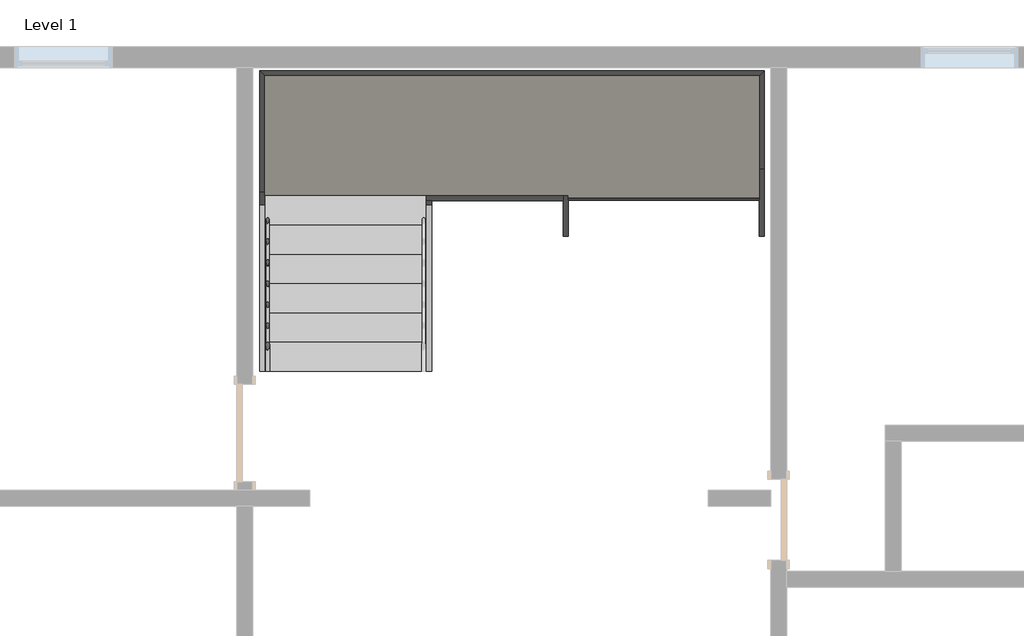
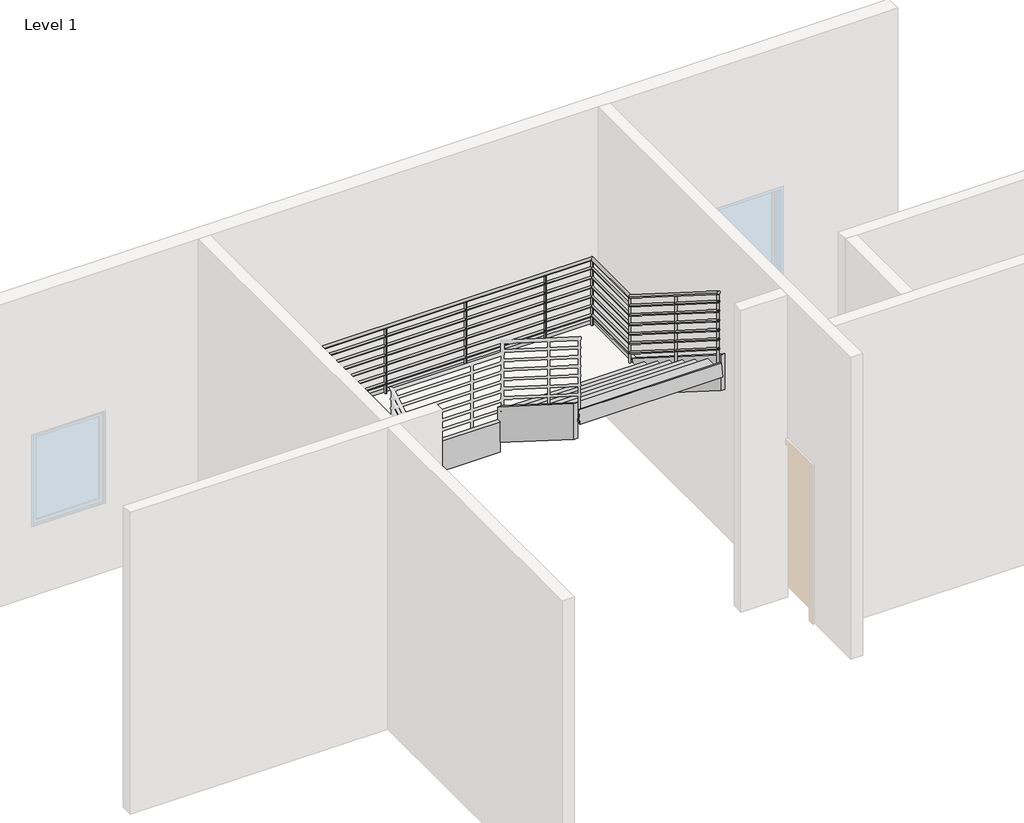
# One storey, part 3 of 3: 8 members, 2 stair flights, 1 railing, 1 slab.
"""IFC4 building model written with IfcOpenShell, lengths in millimetres."""

from ifc_helpers import new_model, si_unit, point, frame, frame_2d, origin, place, context, project, spatial, polyline, circle_curve, ellipse_curve, trimmed, segment, composite_curve, outline, extrude, faceted_brep, transform, mapped, element, save
from ifc_brep_helpers import plane_surface, cylinder_surface, advanced_brep
from components import non_monolithic_landing_b96f42b5, stair_flight_50mm_tread_25mm_nosing_13mm_riser_cb9873a3, stair_flight_50mm_tread_25mm_nosing_13mm_riser_6e0c1f45

model = new_model("IFC4")

# Units and contexts
model_context = context("Model", 3, world=origin())
ifc_project = project(units=[si_unit("LENGTHUNIT", "METRE", prefix="MILLI")], contexts=[model_context])

# Site, building, storey
site = spatial("IfcSite", under=ifc_project)
building = spatial("IfcBuilding", under=site)
storey = spatial("IfcBuildingStorey", under=building, Name="Level 1", Elevation=0.0)

# Members
placement = place(None, origin())
element("IfcMember", 1, ObjectType="Stringer - 50mm Width", at=placement, inside=storey, context=model_context, shape_type="SweptSolid", body=[
    extrude(outline(polyline([(8742.1981148, 0.0), (8742.1981148, 215.089535), (10402.0291183, 1264.7850313), (10517.8981784, 864.7850313), (9150.4568476, 0.0), (8742.1981148, 0.0)])), frame((-2431.5205334, 0.0, 0.0), z_axis=(1.0, 0.0, 0.0), x_axis=(0.0, 1.0, 0.0)), (0.0, 0.0, 1.0), 50.0),
])
element("IfcMember", 2, ObjectType="Stringer - 50mm Width", at=placement, inside=storey, context=model_context, shape_type="SweptSolid", body=[
    extrude(outline(polyline([(8742.1981148, 0.0), (8742.1981148, 215.089535), (10342.1981148, 1226.9472425), (10342.1981148, 753.6703666), (9150.4568476, 0.0), (8742.1981148, 0.0)])), frame((-866.6164824, 0.0, 0.0), z_axis=(1.0, 0.0, 0.0), x_axis=(0.0, 1.0, 0.0)), (0.0, 0.0, 1.0), 50.0),
])
element("IfcMember", 3, ObjectType="Stringer - 50mm Width", at=placement, inside=storey, context=model_context, shape_type="SweptSolid", body=[
    extrude(outline(polyline([(10657.3671112, 1264.7850313), (10541.4980512, 864.7850313), (8742.1981148, 2002.6822243), (8742.1981148, 2475.9591002), (10657.3671112, 1264.7850313)])), frame((2255.6816567, 0.0, 0.0), z_axis=(1.0, 0.0, 0.0), x_axis=(0.0, 1.0, 0.0)), (0.0, 0.0, 1.0), 50.0),
])
element("IfcMember", 4, ObjectType="Stringer - 50mm Width", at=placement, inside=storey, context=model_context, shape_type="SweptSolid", body=[
    extrude(outline(polyline([(10392.1981148, 1432.4808393), (10392.1981148, 959.2039634), (8742.1981148, 2002.6822243), (8742.1981148, 2475.9591002), (10392.1981148, 1432.4808393)])), frame((416.2714992, 0.0, 0.0), z_axis=(1.0, 0.0, 0.0), x_axis=(0.0, 1.0, 0.0)), (0.0, 0.0, 1.0), 50.0),
])
element("IfcMember", 5, ObjectType="Stringer - 50mm Width", at=placement, inside=storey, context=model_context, shape_type="Brep", body=[
    faceted_brep([(2255.6816567, 10657.3671112, 1264.7850313), (2305.6816567, 10657.3671112, 1264.7850313), (2305.6816567, 11563.685068, 1264.7850313), (2255.6816567, 11513.685068, 1264.7850313), (2255.6816567, 10541.4980512, 864.7850313), (2255.6816567, 11513.685068, 864.7850313), (2305.6816567, 10541.4980512, 864.7850313), (2305.6816567, 11563.685068, 864.7850313)], [[[0, 1, 2, 3]], [[4, 0, 3, 5]], [[6, 4, 5, 7]], [[1, 6, 7, 2]], [[2, 7, 5, 3]], [[1, 0, 4, 6]]]),
])
element("IfcMember", 6, ObjectType="Stringer - 50mm Width", at=placement, inside=storey, context=model_context, shape_type="SweptSolid", body=[
    extrude(outline(polyline([(2305.6816567, 11563.685068), (2255.6816567, 11513.685068), (-2381.5205334, 11513.685068), (-2431.5205334, 11563.685068), (2305.6816567, 11563.685068)])), frame((0.0, 0.0, 864.7850313), z_axis=(0.0, 0.0, 1.0), x_axis=(1.0, 0.0, 0.0)), (0.0, 0.0, 1.0), 400.0),
])
element("IfcMember", 7, ObjectType="Stringer - 50mm Width", at=placement, inside=storey, context=model_context, shape_type="Brep", body=[
    faceted_brep([(-2381.5205334, 11513.685068, 1264.7850313), (-2431.5205334, 11563.685068, 1264.7850313), (-2431.5205334, 10402.0291183, 1264.7850313), (-2381.5205334, 10402.0291183, 1264.7850313), (-2381.5205334, 11513.685068, 864.7850313), (-2381.5205334, 10517.8981784, 864.7850313), (-2431.5205334, 11563.685068, 864.7850313), (-2431.5205334, 10517.8981784, 864.7850313)], [[[0, 1, 2, 3]], [[4, 0, 3, 5]], [[6, 4, 5, 7]], [[1, 6, 7, 2]], [[1, 0, 4, 6]], [[2, 7, 5, 3]]]),
])
element("IfcMember", 8, ObjectType="Stringer - 50mm Width", at=placement, inside=storey, context=model_context, shape_type="SweptSolid", body=[
    extrude(outline(polyline([(-866.6164824, 10342.1981148), (-866.6164824, 10392.1981148), (416.2714992, 10392.1981148), (416.2714992, 10342.1981148), (-866.6164824, 10342.1981148)])), frame((0.0, 0.0, 864.7850313), z_axis=(0.0, 0.0, 1.0), x_axis=(1.0, 0.0, 0.0)), (0.0, 0.0, 1.0), 400.0),
])

# Railing
element("IfcRailing", 9, ObjectType="900mm Pipe", at=placement, inside=storey, context=model_context, shape_type="SolidModel", body=[
    advanced_brep(
    [(-2336.1205334, 8742.1981148, 1050.2491997), (-2376.1205334, 8742.1981148, 1050.2491997), (-2336.1205334, 10397.9915678, 2097.3913043), (-2376.1205334, 10397.9915678, 2097.3913043), (-2336.1205334, 11468.285068, 2097.3913043), (-2376.1205334, 11508.285068, 2097.3913043), (2210.2816567, 11468.285068, 2097.3913043), (2250.2816567, 11508.285068, 2097.3913043), (2210.2816567, 10661.4046618, 2097.3913043), (2250.2816567, 10661.4046618, 2097.3913043), (2210.2816567, 8742.1981148, 3311.1187649), (2250.2816567, 8742.1981148, 3311.1187649)],
    [
        (0, 1, ellipse_curve(frame((-2356.1205334, 8742.1981148, 1050.2491997), z_axis=(0.0, -1.0, 0.0), x_axis=(0.0, 0.0, -1.0)), 23.6638438, 20.0)),
        (1, 0, ellipse_curve(frame((-2356.1205334, 8742.1981148, 1050.2491997), z_axis=(0.0, -1.0, 0.0), x_axis=(0.0, 0.0, -1.0)), 23.6638438, 20.0)),
        (0, 2),
        (2, 3, ellipse_curve(frame((-2356.1205334, 10397.9915678, 2097.3913043), z_axis=(0.0, -0.9605132043335073, -0.2782344053149754), x_axis=(0.0, 0.27823440531497523, -0.9605132043335072)), 20.822202, 20.0)),
        (3, 1),
        (3, 2, ellipse_curve(frame((-2356.1205334, 10397.9915678, 2097.3913043), z_axis=(0.0, -0.9605132043335073, -0.2782344053149754), x_axis=(0.0, 0.27823440531497523, -0.9605132043335072)), 20.822202, 20.0)),
        (2, 4),
        (4, 5, ellipse_curve(frame((-2356.1205334, 11488.285068, 2097.3913043), z_axis=(-0.7071067811865483, -0.7071067811865468, 0.0), x_axis=(0.7071067811865468, -0.7071067811865482, 0.0)), 28.2842712, 20.0)),
        (5, 3),
        (5, 4, ellipse_curve(frame((-2356.1205334, 11488.285068, 2097.3913043), z_axis=(-0.7071067811865483, -0.7071067811865468, 0.0), x_axis=(0.7071067811865468, -0.7071067811865482, 0.0)), 28.2842712, 20.0)),
        (4, 6),
        (6, 7, ellipse_curve(frame((2230.2816567, 11488.285068, 2097.3913043), z_axis=(-0.7071067811865468, 0.7071067811865481, 0.0), x_axis=(-0.7071067811865485, -0.7071067811865467, 0.0)), 28.2842712, 20.0)),
        (7, 5),
        (7, 6, ellipse_curve(frame((2230.2816567, 11488.285068, 2097.3913043), z_axis=(-0.7071067811865468, 0.7071067811865481, 0.0), x_axis=(-0.7071067811865485, -0.7071067811865467, 0.0)), 28.2842712, 20.0)),
        (6, 8),
        (8, 9, ellipse_curve(frame((2230.2816567, 10661.4046618, 2097.3913043), z_axis=(0.0, 0.9605132043335073, -0.2782344053149758), x_axis=(0.0, 0.2782344053149754, 0.9605132043335073)), 20.822202, 20.0)),
        (9, 7),
        (9, 8, ellipse_curve(frame((2230.2816567, 10661.4046618, 2097.3913043), z_axis=(0.0, 0.9605132043335073, -0.2782344053149758), x_axis=(0.0, 0.2782344053149754, 0.9605132043335073)), 20.822202, 20.0)),
        (10, 11, ellipse_curve(frame((2230.2816567, 8742.1981148, 3311.1187649), z_axis=(0.0, -1.0, 0.0), x_axis=(0.0, 0.0, -1.0)), 23.6638438, 20.0)),
        (11, 10, ellipse_curve(frame((2230.2816567, 8742.1981148, 3311.1187649), z_axis=(0.0, -1.0, 0.0), x_axis=(0.0, 0.0, -1.0)), 23.6638438, 20.0)),
        (8, 10),
        (11, 9),
    ],
    [
        plane_surface(frame((-2356.1205334, 8742.1981148, 1073.9130435), z_axis=(0.0, -1.0, 0.0), x_axis=(0.0, 0.0, 1.0))),
        cylinder_surface(frame((-2356.1205334, 8752.8880276, 1057.0096189), z_axis=(0.0, -0.8451712313980438, -0.5344956404098299), x_axis=(-1.0, 0.0, 0.0)), 20.0),
        cylinder_surface(frame((-2356.1205334, 10392.1981148, 2097.3913043), z_axis=(0.0, -1.0, 0.0), x_axis=(-1.0, 0.0, 0.0)), 20.0),
        cylinder_surface(frame((-2356.1205334, 11488.285068, 2097.3913043), z_axis=(-1.0, 0.0, 0.0), x_axis=(0.0, 1.0, 0.0)), 20.0),
        cylinder_surface(frame((2230.2816567, 11488.285068, 2097.3913043), z_axis=(0.0, 1.0, 0.0), x_axis=(1.0, 0.0, 0.0)), 20.0),
        plane_surface(frame((2230.2816567, 8742.1981148, 3334.7826087), z_axis=(0.0, -1.0, 0.0), x_axis=(0.0, 0.0, -1.0))),
        cylinder_surface(frame((2230.2816567, 10656.508202, 2100.4878797), z_axis=(0.0, 0.8451712313980435, -0.5344956404098304), x_axis=(1.0, 0.0, 0.0)), 20.0),
    ],
    [
        (0, [[1, 2]]),
        (1, [[-1, 3, 4, 5]]),
        (1, [[-2, -5, 6, -3]]),
        (2, [[-4, 7, 8, 9]]),
        (2, [[-6, -9, 10, -7]]),
        (3, [[-8, 11, 12, 13]]),
        (3, [[-10, -13, 14, -11]]),
        (4, [[-12, 15, 16, 17]]),
        (4, [[-14, -17, 18, -15]]),
        (5, [[19, 20]]),
        (6, [[-16, 21, -20, 22]]),
        (6, [[-18, -22, -19, -21]]),
    ],
),
    advanced_brep(
    [(-2341.1205334, 8742.1981148, 931.1651606), (-2371.1205334, 8742.1981148, 931.1651606), (-2341.1205334, 10396.5432045, 1977.3913043), (-2371.1205334, 10396.5432045, 1977.3913043), (-2341.1205334, 11473.285068, 1977.3913043), (-2371.1205334, 11503.285068, 1977.3913043), (2215.2816567, 11473.285068, 1977.3913043), (2245.2816567, 11503.285068, 1977.3913043), (2215.2816567, 10662.853025, 1977.3913043), (2245.2816567, 10662.853025, 1977.3913043), (2215.2816567, 8742.1981148, 3192.0347258), (2245.2816567, 8742.1981148, 3192.0347258)],
    [
        (0, 1, ellipse_curve(frame((-2356.1205334, 8742.1981148, 931.1651606), z_axis=(0.0, -1.0, 0.0), x_axis=(0.0, 0.0, -1.0)), 17.7478828, 15.0)),
        (1, 0, ellipse_curve(frame((-2356.1205334, 8742.1981148, 931.1651606), z_axis=(0.0, -1.0, 0.0), x_axis=(0.0, 0.0, -1.0)), 17.7478828, 15.0)),
        (0, 2),
        (2, 3, ellipse_curve(frame((-2356.1205334, 10396.5432045, 1977.3913043), z_axis=(0.0, -0.9605132043335073, -0.2782344053149755), x_axis=(0.0, 0.27823440531497556, -0.9605132043335073)), 15.6166515, 15.0)),
        (3, 1),
        (3, 2, ellipse_curve(frame((-2356.1205334, 10396.5432045, 1977.3913043), z_axis=(0.0, -0.9605132043335073, -0.2782344053149755), x_axis=(0.0, 0.27823440531497556, -0.9605132043335073)), 15.6166515, 15.0)),
        (2, 4),
        (4, 5, ellipse_curve(frame((-2356.1205334, 11488.285068, 1977.3913043), z_axis=(-0.7071067811865483, -0.7071067811865468, 0.0), x_axis=(0.7071067811865468, -0.7071067811865482, 0.0)), 21.2132034, 15.0)),
        (5, 3),
        (5, 4, ellipse_curve(frame((-2356.1205334, 11488.285068, 1977.3913043), z_axis=(-0.7071067811865483, -0.7071067811865468, 0.0), x_axis=(0.7071067811865468, -0.7071067811865482, 0.0)), 21.2132034, 15.0)),
        (4, 6),
        (6, 7, ellipse_curve(frame((2230.2816567, 11488.285068, 1977.3913043), z_axis=(-0.7071067811865468, 0.7071067811865481, 0.0), x_axis=(-0.7071067811865485, -0.7071067811865467, 0.0)), 21.2132034, 15.0)),
        (7, 5),
        (7, 6, ellipse_curve(frame((2230.2816567, 11488.285068, 1977.3913043), z_axis=(-0.7071067811865468, 0.7071067811865481, 0.0), x_axis=(-0.7071067811865485, -0.7071067811865467, 0.0)), 21.2132034, 15.0)),
        (6, 8),
        (8, 9, ellipse_curve(frame((2230.2816567, 10662.853025, 1977.3913043), z_axis=(0.0, 0.9605132043335073, -0.27823440531497573), x_axis=(0.0, 0.27823440531497545, 0.9605132043335072)), 15.6166515, 15.0)),
        (9, 7),
        (9, 8, ellipse_curve(frame((2230.2816567, 10662.853025, 1977.3913043), z_axis=(0.0, 0.9605132043335073, -0.27823440531497573), x_axis=(0.0, 0.27823440531497545, 0.9605132043335072)), 15.6166515, 15.0)),
        (10, 11, ellipse_curve(frame((2230.2816567, 8742.1981148, 3192.0347258), z_axis=(0.0, -1.0, 0.0), x_axis=(0.0, 0.0, -1.0)), 17.7478828, 15.0)),
        (11, 10, ellipse_curve(frame((2230.2816567, 8742.1981148, 3192.0347258), z_axis=(0.0, -1.0, 0.0), x_axis=(0.0, 0.0, -1.0)), 17.7478828, 15.0)),
        (8, 10),
        (11, 9),
    ],
    [
        plane_surface(frame((-2356.1205334, 8742.1981148, 948.9130435), z_axis=(0.0, -1.0, 0.0), x_axis=(0.0, 0.0, 1.0))),
        cylinder_surface(frame((-2356.1205334, 8750.2155494, 936.235475), z_axis=(0.0, -0.8451712313980438, -0.5344956404098301), x_axis=(-1.0, 0.0, 0.0)), 15.0),
        cylinder_surface(frame((-2356.1205334, 10392.1981148, 1977.3913043), z_axis=(0.0, -1.0, 0.0), x_axis=(-1.0, 0.0, 0.0)), 15.0),
        cylinder_surface(frame((-2356.1205334, 11488.285068, 1977.3913043), z_axis=(-1.0, 0.0, 0.0), x_axis=(0.0, 1.0, 0.0)), 15.0),
        cylinder_surface(frame((2230.2816567, 11488.285068, 1977.3913043), z_axis=(0.0, 1.0, 0.0), x_axis=(1.0, 0.0, 0.0)), 15.0),
        plane_surface(frame((2230.2816567, 8742.1981148, 3209.7826087), z_axis=(0.0, -1.0, 0.0), x_axis=(0.0, 0.0, -1.0))),
        cylinder_surface(frame((2230.2816567, 10659.1806802, 1979.7137359), z_axis=(0.0, 0.8451712313980436, -0.5344956404098303), x_axis=(1.0, 0.0, 0.0)), 15.0),
    ],
    [
        (0, [[1, 2]]),
        (1, [[-1, 3, 4, 5]]),
        (1, [[-2, -5, 6, -3]]),
        (2, [[-4, 7, 8, 9]]),
        (2, [[-6, -9, 10, -7]]),
        (3, [[-8, 11, 12, 13]]),
        (3, [[-10, -13, 14, -11]]),
        (4, [[-12, 15, 16, 17]]),
        (4, [[-14, -17, 18, -15]]),
        (5, [[19, 20]]),
        (6, [[-16, 21, -20, 22]]),
        (6, [[-18, -22, -19, -21]]),
    ],
),
    advanced_brep(
    [(-2341.1205334, 8742.1981148, 806.1651606), (-2371.1205334, 8742.1981148, 806.1651606), (-2341.1205334, 10396.5432045, 1852.3913043), (-2371.1205334, 10396.5432045, 1852.3913043), (-2341.1205334, 11473.285068, 1852.3913043), (-2371.1205334, 11503.285068, 1852.3913043), (2215.2816567, 11473.285068, 1852.3913043), (2245.2816567, 11503.285068, 1852.3913043), (2215.2816567, 10662.853025, 1852.3913043), (2245.2816567, 10662.853025, 1852.3913043), (2215.2816567, 8742.1981148, 3067.0347258), (2245.2816567, 8742.1981148, 3067.0347258)],
    [
        (0, 1, ellipse_curve(frame((-2356.1205334, 8742.1981148, 806.1651606), z_axis=(0.0, -1.0, 0.0), x_axis=(0.0, 0.0, -1.0)), 17.7478828, 15.0)),
        (1, 0, ellipse_curve(frame((-2356.1205334, 8742.1981148, 806.1651606), z_axis=(0.0, -1.0, 0.0), x_axis=(0.0, 0.0, -1.0)), 17.7478828, 15.0)),
        (0, 2),
        (2, 3, ellipse_curve(frame((-2356.1205334, 10396.5432045, 1852.3913043), z_axis=(0.0, -0.9605132043335073, -0.2782344053149755), x_axis=(0.0, 0.27823440531497556, -0.9605132043335073)), 15.6166515, 15.0)),
        (3, 1),
        (3, 2, ellipse_curve(frame((-2356.1205334, 10396.5432045, 1852.3913043), z_axis=(0.0, -0.9605132043335073, -0.2782344053149755), x_axis=(0.0, 0.27823440531497556, -0.9605132043335073)), 15.6166515, 15.0)),
        (2, 4),
        (4, 5, ellipse_curve(frame((-2356.1205334, 11488.285068, 1852.3913043), z_axis=(-0.7071067811865483, -0.7071067811865468, 0.0), x_axis=(0.7071067811865468, -0.7071067811865482, 0.0)), 21.2132034, 15.0)),
        (5, 3),
        (5, 4, ellipse_curve(frame((-2356.1205334, 11488.285068, 1852.3913043), z_axis=(-0.7071067811865483, -0.7071067811865468, 0.0), x_axis=(0.7071067811865468, -0.7071067811865482, 0.0)), 21.2132034, 15.0)),
        (4, 6),
        (6, 7, ellipse_curve(frame((2230.2816567, 11488.285068, 1852.3913043), z_axis=(-0.7071067811865468, 0.7071067811865481, 0.0), x_axis=(-0.7071067811865485, -0.7071067811865467, 0.0)), 21.2132034, 15.0)),
        (7, 5),
        (7, 6, ellipse_curve(frame((2230.2816567, 11488.285068, 1852.3913043), z_axis=(-0.7071067811865468, 0.7071067811865481, 0.0), x_axis=(-0.7071067811865485, -0.7071067811865467, 0.0)), 21.2132034, 15.0)),
        (6, 8),
        (8, 9, ellipse_curve(frame((2230.2816567, 10662.853025, 1852.3913043), z_axis=(0.0, 0.9605132043335073, -0.27823440531497573), x_axis=(0.0, 0.27823440531497545, 0.9605132043335072)), 15.6166515, 15.0)),
        (9, 7),
        (9, 8, ellipse_curve(frame((2230.2816567, 10662.853025, 1852.3913043), z_axis=(0.0, 0.9605132043335073, -0.27823440531497573), x_axis=(0.0, 0.27823440531497545, 0.9605132043335072)), 15.6166515, 15.0)),
        (10, 11, ellipse_curve(frame((2230.2816567, 8742.1981148, 3067.0347258), z_axis=(0.0, -1.0, 0.0), x_axis=(0.0, 0.0, -1.0)), 17.7478828, 15.0)),
        (11, 10, ellipse_curve(frame((2230.2816567, 8742.1981148, 3067.0347258), z_axis=(0.0, -1.0, 0.0), x_axis=(0.0, 0.0, -1.0)), 17.7478828, 15.0)),
        (8, 10),
        (11, 9),
    ],
    [
        plane_surface(frame((-2356.1205334, 8742.1981148, 823.9130435), z_axis=(0.0, -1.0, 0.0), x_axis=(0.0, 0.0, 1.0))),
        cylinder_surface(frame((-2356.1205334, 8750.2155494, 811.235475), z_axis=(0.0, -0.8451712313980438, -0.5344956404098301), x_axis=(-1.0, 0.0, 0.0)), 15.0),
        cylinder_surface(frame((-2356.1205334, 10392.1981148, 1852.3913043), z_axis=(0.0, -1.0, 0.0), x_axis=(-1.0, 0.0, 0.0)), 15.0),
        cylinder_surface(frame((-2356.1205334, 11488.285068, 1852.3913043), z_axis=(-1.0, 0.0, 0.0), x_axis=(0.0, 1.0, 0.0)), 15.0),
        cylinder_surface(frame((2230.2816567, 11488.285068, 1852.3913043), z_axis=(0.0, 1.0, 0.0), x_axis=(1.0, 0.0, 0.0)), 15.0),
        plane_surface(frame((2230.2816567, 8742.1981148, 3084.7826087), z_axis=(0.0, -1.0, 0.0), x_axis=(0.0, 0.0, -1.0))),
        cylinder_surface(frame((2230.2816567, 10659.1806802, 1854.7137359), z_axis=(0.0, 0.8451712313980436, -0.5344956404098303), x_axis=(1.0, 0.0, 0.0)), 15.0),
    ],
    [
        (0, [[1, 2]]),
        (1, [[-1, 3, 4, 5]]),
        (1, [[-2, -5, 6, -3]]),
        (2, [[-4, 7, 8, 9]]),
        (2, [[-6, -9, 10, -7]]),
        (3, [[-8, 11, 12, 13]]),
        (3, [[-10, -13, 14, -11]]),
        (4, [[-12, 15, 16, 17]]),
        (4, [[-14, -17, 18, -15]]),
        (5, [[19, 20]]),
        (6, [[-16, 21, -20, 22]]),
        (6, [[-18, -22, -19, -21]]),
    ],
),
    advanced_brep(
    [(-2341.1205334, 8742.1981148, 681.1651606), (-2371.1205334, 8742.1981148, 681.1651606), (-2341.1205334, 10396.5432045, 1727.3913043), (-2371.1205334, 10396.5432045, 1727.3913043), (-2341.1205334, 11473.285068, 1727.3913043), (-2371.1205334, 11503.285068, 1727.3913043), (2215.2816567, 11473.285068, 1727.3913043), (2245.2816567, 11503.285068, 1727.3913043), (2215.2816567, 10662.853025, 1727.3913043), (2245.2816567, 10662.853025, 1727.3913043), (2215.2816567, 8742.1981148, 2942.0347258), (2245.2816567, 8742.1981148, 2942.0347258)],
    [
        (0, 1, ellipse_curve(frame((-2356.1205334, 8742.1981148, 681.1651606), z_axis=(0.0, -1.0, 0.0), x_axis=(0.0, 0.0, -1.0)), 17.7478828, 15.0)),
        (1, 0, ellipse_curve(frame((-2356.1205334, 8742.1981148, 681.1651606), z_axis=(0.0, -1.0, 0.0), x_axis=(0.0, 0.0, -1.0)), 17.7478828, 15.0)),
        (0, 2),
        (2, 3, ellipse_curve(frame((-2356.1205334, 10396.5432045, 1727.3913043), z_axis=(0.0, -0.9605132043335073, -0.2782344053149755), x_axis=(0.0, 0.27823440531497556, -0.9605132043335073)), 15.6166515, 15.0)),
        (3, 1),
        (3, 2, ellipse_curve(frame((-2356.1205334, 10396.5432045, 1727.3913043), z_axis=(0.0, -0.9605132043335073, -0.2782344053149755), x_axis=(0.0, 0.27823440531497556, -0.9605132043335073)), 15.6166515, 15.0)),
        (2, 4),
        (4, 5, ellipse_curve(frame((-2356.1205334, 11488.285068, 1727.3913043), z_axis=(-0.7071067811865483, -0.7071067811865468, 0.0), x_axis=(0.7071067811865468, -0.7071067811865482, 0.0)), 21.2132034, 15.0)),
        (5, 3),
        (5, 4, ellipse_curve(frame((-2356.1205334, 11488.285068, 1727.3913043), z_axis=(-0.7071067811865483, -0.7071067811865468, 0.0), x_axis=(0.7071067811865468, -0.7071067811865482, 0.0)), 21.2132034, 15.0)),
        (4, 6),
        (6, 7, ellipse_curve(frame((2230.2816567, 11488.285068, 1727.3913043), z_axis=(-0.7071067811865468, 0.7071067811865481, 0.0), x_axis=(-0.7071067811865485, -0.7071067811865467, 0.0)), 21.2132034, 15.0)),
        (7, 5),
        (7, 6, ellipse_curve(frame((2230.2816567, 11488.285068, 1727.3913043), z_axis=(-0.7071067811865468, 0.7071067811865481, 0.0), x_axis=(-0.7071067811865485, -0.7071067811865467, 0.0)), 21.2132034, 15.0)),
        (6, 8),
        (8, 9, ellipse_curve(frame((2230.2816567, 10662.853025, 1727.3913043), z_axis=(0.0, 0.9605132043335073, -0.2782344053149758), x_axis=(0.0, 0.2782344053149754, 0.9605132043335073)), 15.6166515, 15.0)),
        (9, 7),
        (9, 8, ellipse_curve(frame((2230.2816567, 10662.853025, 1727.3913043), z_axis=(0.0, 0.9605132043335073, -0.2782344053149758), x_axis=(0.0, 0.2782344053149754, 0.9605132043335073)), 15.6166515, 15.0)),
        (10, 11, ellipse_curve(frame((2230.2816567, 8742.1981148, 2942.0347258), z_axis=(0.0, -1.0, 0.0), x_axis=(0.0, 0.0, -1.0)), 17.7478828, 15.0)),
        (11, 10, ellipse_curve(frame((2230.2816567, 8742.1981148, 2942.0347258), z_axis=(0.0, -1.0, 0.0), x_axis=(0.0, 0.0, -1.0)), 17.7478828, 15.0)),
        (8, 10),
        (11, 9),
    ],
    [
        plane_surface(frame((-2356.1205334, 8742.1981148, 698.9130435), z_axis=(0.0, -1.0, 0.0), x_axis=(0.0, 0.0, 1.0))),
        cylinder_surface(frame((-2356.1205334, 8750.2155494, 686.235475), z_axis=(0.0, -0.8451712313980438, -0.5344956404098301), x_axis=(-1.0, 0.0, 0.0)), 15.0),
        cylinder_surface(frame((-2356.1205334, 10392.1981148, 1727.3913043), z_axis=(0.0, -1.0, 0.0), x_axis=(-1.0, 0.0, 0.0)), 15.0),
        cylinder_surface(frame((-2356.1205334, 11488.285068, 1727.3913043), z_axis=(-1.0, 0.0, 0.0), x_axis=(0.0, 1.0, 0.0)), 15.0),
        cylinder_surface(frame((2230.2816567, 11488.285068, 1727.3913043), z_axis=(0.0, 1.0, 0.0), x_axis=(1.0, 0.0, 0.0)), 15.0),
        plane_surface(frame((2230.2816567, 8742.1981148, 2959.7826087), z_axis=(0.0, -1.0, 0.0), x_axis=(0.0, 0.0, -1.0))),
        cylinder_surface(frame((2230.2816567, 10659.1806802, 1729.7137359), z_axis=(0.0, 0.8451712313980435, -0.5344956404098304), x_axis=(1.0, 0.0, 0.0)), 15.0),
    ],
    [
        (0, [[1, 2]]),
        (1, [[-1, 3, 4, 5]]),
        (1, [[-2, -5, 6, -3]]),
        (2, [[-4, 7, 8, 9]]),
        (2, [[-6, -9, 10, -7]]),
        (3, [[-8, 11, 12, 13]]),
        (3, [[-10, -13, 14, -11]]),
        (4, [[-12, 15, 16, 17]]),
        (4, [[-14, -17, 18, -15]]),
        (5, [[19, 20]]),
        (6, [[-16, 21, -20, 22]]),
        (6, [[-18, -22, -19, -21]]),
    ],
),
    advanced_brep(
    [(-2341.1205334, 8742.1981148, 556.1651606), (-2371.1205334, 8742.1981148, 556.1651606), (-2341.1205334, 10396.5432045, 1602.3913043), (-2371.1205334, 10396.5432045, 1602.3913043), (-2341.1205334, 11473.285068, 1602.3913043), (-2371.1205334, 11503.285068, 1602.3913043), (2215.2816567, 11473.285068, 1602.3913043), (2245.2816567, 11503.285068, 1602.3913043), (2215.2816567, 10662.853025, 1602.3913043), (2245.2816567, 10662.853025, 1602.3913043), (2215.2816567, 8742.1981148, 2817.0347258), (2245.2816567, 8742.1981148, 2817.0347258)],
    [
        (0, 1, ellipse_curve(frame((-2356.1205334, 8742.1981148, 556.1651606), z_axis=(0.0, -1.0, 0.0), x_axis=(0.0, 0.0, -1.0)), 17.7478828, 15.0)),
        (1, 0, ellipse_curve(frame((-2356.1205334, 8742.1981148, 556.1651606), z_axis=(0.0, -1.0, 0.0), x_axis=(0.0, 0.0, -1.0)), 17.7478828, 15.0)),
        (0, 2),
        (2, 3, ellipse_curve(frame((-2356.1205334, 10396.5432045, 1602.3913043), z_axis=(0.0, -0.9605132043335073, -0.2782344053149755), x_axis=(0.0, 0.27823440531497556, -0.9605132043335073)), 15.6166515, 15.0)),
        (3, 1),
        (3, 2, ellipse_curve(frame((-2356.1205334, 10396.5432045, 1602.3913043), z_axis=(0.0, -0.9605132043335073, -0.2782344053149755), x_axis=(0.0, 0.27823440531497556, -0.9605132043335073)), 15.6166515, 15.0)),
        (2, 4),
        (4, 5, ellipse_curve(frame((-2356.1205334, 11488.285068, 1602.3913043), z_axis=(-0.7071067811865483, -0.7071067811865468, 0.0), x_axis=(0.7071067811865468, -0.7071067811865482, 0.0)), 21.2132034, 15.0)),
        (5, 3),
        (5, 4, ellipse_curve(frame((-2356.1205334, 11488.285068, 1602.3913043), z_axis=(-0.7071067811865483, -0.7071067811865468, 0.0), x_axis=(0.7071067811865468, -0.7071067811865482, 0.0)), 21.2132034, 15.0)),
        (4, 6),
        (6, 7, ellipse_curve(frame((2230.2816567, 11488.285068, 1602.3913043), z_axis=(-0.7071067811865468, 0.7071067811865481, 0.0), x_axis=(-0.7071067811865485, -0.7071067811865467, 0.0)), 21.2132034, 15.0)),
        (7, 5),
        (7, 6, ellipse_curve(frame((2230.2816567, 11488.285068, 1602.3913043), z_axis=(-0.7071067811865468, 0.7071067811865481, 0.0), x_axis=(-0.7071067811865485, -0.7071067811865467, 0.0)), 21.2132034, 15.0)),
        (6, 8),
        (8, 9, ellipse_curve(frame((2230.2816567, 10662.853025, 1602.3913043), z_axis=(0.0, 0.9605132043335073, -0.27823440531497573), x_axis=(0.0, 0.27823440531497545, 0.9605132043335072)), 15.6166515, 15.0)),
        (9, 7),
        (9, 8, ellipse_curve(frame((2230.2816567, 10662.853025, 1602.3913043), z_axis=(0.0, 0.9605132043335073, -0.27823440531497573), x_axis=(0.0, 0.27823440531497545, 0.9605132043335072)), 15.6166515, 15.0)),
        (10, 11, ellipse_curve(frame((2230.2816567, 8742.1981148, 2817.0347258), z_axis=(0.0, -1.0, 0.0), x_axis=(0.0, 0.0, -1.0)), 17.7478828, 15.0)),
        (11, 10, ellipse_curve(frame((2230.2816567, 8742.1981148, 2817.0347258), z_axis=(0.0, -1.0, 0.0), x_axis=(0.0, 0.0, -1.0)), 17.7478828, 15.0)),
        (8, 10),
        (11, 9),
    ],
    [
        plane_surface(frame((-2356.1205334, 8742.1981148, 573.9130435), z_axis=(0.0, -1.0, 0.0), x_axis=(0.0, 0.0, 1.0))),
        cylinder_surface(frame((-2356.1205334, 8750.2155494, 561.235475), z_axis=(0.0, -0.8451712313980438, -0.5344956404098301), x_axis=(-1.0, 0.0, 0.0)), 15.0),
        cylinder_surface(frame((-2356.1205334, 10392.1981148, 1602.3913043), z_axis=(0.0, -1.0, 0.0), x_axis=(-1.0, 0.0, 0.0)), 15.0),
        cylinder_surface(frame((-2356.1205334, 11488.285068, 1602.3913043), z_axis=(-1.0, 0.0, 0.0), x_axis=(0.0, 1.0, 0.0)), 15.0),
        cylinder_surface(frame((2230.2816567, 11488.285068, 1602.3913043), z_axis=(0.0, 1.0, 0.0), x_axis=(1.0, 0.0, 0.0)), 15.0),
        plane_surface(frame((2230.2816567, 8742.1981148, 2834.7826087), z_axis=(0.0, -1.0, 0.0), x_axis=(0.0, 0.0, -1.0))),
        cylinder_surface(frame((2230.2816567, 10659.1806802, 1604.7137359), z_axis=(0.0, 0.8451712313980436, -0.5344956404098303), x_axis=(1.0, 0.0, 0.0)), 15.0),
    ],
    [
        (0, [[1, 2]]),
        (1, [[-1, 3, 4, 5]]),
        (1, [[-2, -5, 6, -3]]),
        (2, [[-4, 7, 8, 9]]),
        (2, [[-6, -9, 10, -7]]),
        (3, [[-8, 11, 12, 13]]),
        (3, [[-10, -13, 14, -11]]),
        (4, [[-12, 15, 16, 17]]),
        (4, [[-14, -17, 18, -15]]),
        (5, [[19, 20]]),
        (6, [[-16, 21, -20, 22]]),
        (6, [[-18, -22, -19, -21]]),
    ],
),
    advanced_brep(
    [(-2341.1205334, 8742.1981148, 431.1651606), (-2371.1205334, 8742.1981148, 431.1651606), (-2341.1205334, 10396.5432045, 1477.3913043), (-2371.1205334, 10396.5432045, 1477.3913043), (-2341.1205334, 11473.285068, 1477.3913043), (-2371.1205334, 11503.285068, 1477.3913043), (2215.2816567, 11473.285068, 1477.3913043), (2245.2816567, 11503.285068, 1477.3913043), (2215.2816567, 10662.853025, 1477.3913043), (2245.2816567, 10662.853025, 1477.3913043), (2215.2816567, 8742.1981148, 2692.0347258), (2245.2816567, 8742.1981148, 2692.0347258)],
    [
        (0, 1, ellipse_curve(frame((-2356.1205334, 8742.1981148, 431.1651606), z_axis=(0.0, -1.0, 0.0), x_axis=(0.0, 0.0, -1.0)), 17.7478828, 15.0)),
        (1, 0, ellipse_curve(frame((-2356.1205334, 8742.1981148, 431.1651606), z_axis=(0.0, -1.0, 0.0), x_axis=(0.0, 0.0, -1.0)), 17.7478828, 15.0)),
        (0, 2),
        (2, 3, ellipse_curve(frame((-2356.1205334, 10396.5432045, 1477.3913043), z_axis=(0.0, -0.9605132043335073, -0.2782344053149755), x_axis=(0.0, 0.27823440531497556, -0.9605132043335073)), 15.6166515, 15.0)),
        (3, 1),
        (3, 2, ellipse_curve(frame((-2356.1205334, 10396.5432045, 1477.3913043), z_axis=(0.0, -0.9605132043335073, -0.2782344053149755), x_axis=(0.0, 0.27823440531497556, -0.9605132043335073)), 15.6166515, 15.0)),
        (2, 4),
        (4, 5, ellipse_curve(frame((-2356.1205334, 11488.285068, 1477.3913043), z_axis=(-0.7071067811865483, -0.7071067811865468, 0.0), x_axis=(0.7071067811865468, -0.7071067811865482, 0.0)), 21.2132034, 15.0)),
        (5, 3),
        (5, 4, ellipse_curve(frame((-2356.1205334, 11488.285068, 1477.3913043), z_axis=(-0.7071067811865483, -0.7071067811865468, 0.0), x_axis=(0.7071067811865468, -0.7071067811865482, 0.0)), 21.2132034, 15.0)),
        (4, 6),
        (6, 7, ellipse_curve(frame((2230.2816567, 11488.285068, 1477.3913043), z_axis=(-0.7071067811865468, 0.7071067811865481, 0.0), x_axis=(-0.7071067811865485, -0.7071067811865467, 0.0)), 21.2132034, 15.0)),
        (7, 5),
        (7, 6, ellipse_curve(frame((2230.2816567, 11488.285068, 1477.3913043), z_axis=(-0.7071067811865468, 0.7071067811865481, 0.0), x_axis=(-0.7071067811865485, -0.7071067811865467, 0.0)), 21.2132034, 15.0)),
        (6, 8),
        (8, 9, ellipse_curve(frame((2230.2816567, 10662.853025, 1477.3913043), z_axis=(0.0, 0.9605132043335073, -0.27823440531497573), x_axis=(0.0, 0.27823440531497545, 0.9605132043335072)), 15.6166515, 15.0)),
        (9, 7),
        (9, 8, ellipse_curve(frame((2230.2816567, 10662.853025, 1477.3913043), z_axis=(0.0, 0.9605132043335073, -0.27823440531497573), x_axis=(0.0, 0.27823440531497545, 0.9605132043335072)), 15.6166515, 15.0)),
        (10, 11, ellipse_curve(frame((2230.2816567, 8742.1981148, 2692.0347258), z_axis=(0.0, -1.0, 0.0), x_axis=(0.0, 0.0, -1.0)), 17.7478828, 15.0)),
        (11, 10, ellipse_curve(frame((2230.2816567, 8742.1981148, 2692.0347258), z_axis=(0.0, -1.0, 0.0), x_axis=(0.0, 0.0, -1.0)), 17.7478828, 15.0)),
        (8, 10),
        (11, 9),
    ],
    [
        plane_surface(frame((-2356.1205334, 8742.1981148, 448.9130435), z_axis=(0.0, -1.0, 0.0), x_axis=(0.0, 0.0, 1.0))),
        cylinder_surface(frame((-2356.1205334, 8750.2155494, 436.235475), z_axis=(0.0, -0.8451712313980438, -0.5344956404098301), x_axis=(-1.0, 0.0, 0.0)), 15.0),
        cylinder_surface(frame((-2356.1205334, 10392.1981148, 1477.3913043), z_axis=(0.0, -1.0, 0.0), x_axis=(-1.0, 0.0, 0.0)), 15.0),
        cylinder_surface(frame((-2356.1205334, 11488.285068, 1477.3913043), z_axis=(-1.0, 0.0, 0.0), x_axis=(0.0, 1.0, 0.0)), 15.0),
        cylinder_surface(frame((2230.2816567, 11488.285068, 1477.3913043), z_axis=(0.0, 1.0, 0.0), x_axis=(1.0, 0.0, 0.0)), 15.0),
        plane_surface(frame((2230.2816567, 8742.1981148, 2709.7826087), z_axis=(0.0, -1.0, 0.0), x_axis=(0.0, 0.0, -1.0))),
        cylinder_surface(frame((2230.2816567, 10659.1806802, 1479.7137359), z_axis=(0.0, 0.8451712313980436, -0.5344956404098303), x_axis=(1.0, 0.0, 0.0)), 15.0),
    ],
    [
        (0, [[1, 2]]),
        (1, [[-1, 3, 4, 5]]),
        (1, [[-2, -5, 6, -3]]),
        (2, [[-4, 7, 8, 9]]),
        (2, [[-6, -9, 10, -7]]),
        (3, [[-8, 11, 12, 13]]),
        (3, [[-10, -13, 14, -11]]),
        (4, [[-12, 15, 16, 17]]),
        (4, [[-14, -17, 18, -15]]),
        (5, [[19, 20]]),
        (6, [[-16, 21, -20, 22]]),
        (6, [[-18, -22, -19, -21]]),
    ],
),
    advanced_brep(
    [(-2341.1205334, 8742.1981148, 306.1651606), (-2371.1205334, 8742.1981148, 306.1651606), (-2341.1205334, 10396.5432045, 1352.3913043), (-2371.1205334, 10396.5432045, 1352.3913043), (-2341.1205334, 11473.285068, 1352.3913043), (-2371.1205334, 11503.285068, 1352.3913043), (2215.2816567, 11473.285068, 1352.3913043), (2245.2816567, 11503.285068, 1352.3913043), (2215.2816567, 10662.853025, 1352.3913043), (2245.2816567, 10662.853025, 1352.3913043), (2215.2816567, 8742.1981148, 2567.0347258), (2245.2816567, 8742.1981148, 2567.0347258)],
    [
        (0, 1, ellipse_curve(frame((-2356.1205334, 8742.1981148, 306.1651606), z_axis=(0.0, -1.0, 0.0), x_axis=(0.0, 0.0, -1.0)), 17.7478828, 15.0)),
        (1, 0, ellipse_curve(frame((-2356.1205334, 8742.1981148, 306.1651606), z_axis=(0.0, -1.0, 0.0), x_axis=(0.0, 0.0, -1.0)), 17.7478828, 15.0)),
        (0, 2),
        (2, 3, ellipse_curve(frame((-2356.1205334, 10396.5432045, 1352.3913043), z_axis=(0.0, -0.9605132043335073, -0.2782344053149755), x_axis=(0.0, 0.27823440531497556, -0.9605132043335073)), 15.6166515, 15.0)),
        (3, 1),
        (3, 2, ellipse_curve(frame((-2356.1205334, 10396.5432045, 1352.3913043), z_axis=(0.0, -0.9605132043335073, -0.2782344053149755), x_axis=(0.0, 0.27823440531497556, -0.9605132043335073)), 15.6166515, 15.0)),
        (2, 4),
        (4, 5, ellipse_curve(frame((-2356.1205334, 11488.285068, 1352.3913043), z_axis=(-0.7071067811865483, -0.7071067811865468, 0.0), x_axis=(0.7071067811865468, -0.7071067811865482, 0.0)), 21.2132034, 15.0)),
        (5, 3),
        (5, 4, ellipse_curve(frame((-2356.1205334, 11488.285068, 1352.3913043), z_axis=(-0.7071067811865483, -0.7071067811865468, 0.0), x_axis=(0.7071067811865468, -0.7071067811865482, 0.0)), 21.2132034, 15.0)),
        (4, 6),
        (6, 7, ellipse_curve(frame((2230.2816567, 11488.285068, 1352.3913043), z_axis=(-0.7071067811865468, 0.7071067811865481, 0.0), x_axis=(-0.7071067811865485, -0.7071067811865467, 0.0)), 21.2132034, 15.0)),
        (7, 5),
        (7, 6, ellipse_curve(frame((2230.2816567, 11488.285068, 1352.3913043), z_axis=(-0.7071067811865468, 0.7071067811865481, 0.0), x_axis=(-0.7071067811865485, -0.7071067811865467, 0.0)), 21.2132034, 15.0)),
        (6, 8),
        (8, 9, ellipse_curve(frame((2230.2816567, 10662.853025, 1352.3913043), z_axis=(0.0, 0.9605132043335073, -0.27823440531497573), x_axis=(0.0, 0.27823440531497545, 0.9605132043335072)), 15.6166515, 15.0)),
        (9, 7),
        (9, 8, ellipse_curve(frame((2230.2816567, 10662.853025, 1352.3913043), z_axis=(0.0, 0.9605132043335073, -0.27823440531497573), x_axis=(0.0, 0.27823440531497545, 0.9605132043335072)), 15.6166515, 15.0)),
        (10, 11, ellipse_curve(frame((2230.2816567, 8742.1981148, 2567.0347258), z_axis=(0.0, -1.0, 0.0), x_axis=(0.0, 0.0, -1.0)), 17.7478828, 15.0)),
        (11, 10, ellipse_curve(frame((2230.2816567, 8742.1981148, 2567.0347258), z_axis=(0.0, -1.0, 0.0), x_axis=(0.0, 0.0, -1.0)), 17.7478828, 15.0)),
        (8, 10),
        (11, 9),
    ],
    [
        plane_surface(frame((-2356.1205334, 8742.1981148, 323.9130435), z_axis=(0.0, -1.0, 0.0), x_axis=(0.0, 0.0, 1.0))),
        cylinder_surface(frame((-2356.1205334, 8750.2155494, 311.235475), z_axis=(0.0, -0.8451712313980438, -0.5344956404098301), x_axis=(-1.0, 0.0, 0.0)), 15.0),
        cylinder_surface(frame((-2356.1205334, 10392.1981148, 1352.3913043), z_axis=(0.0, -1.0, 0.0), x_axis=(-1.0, 0.0, 0.0)), 15.0),
        cylinder_surface(frame((-2356.1205334, 11488.285068, 1352.3913043), z_axis=(-1.0, 0.0, 0.0), x_axis=(0.0, 1.0, 0.0)), 15.0),
        cylinder_surface(frame((2230.2816567, 11488.285068, 1352.3913043), z_axis=(0.0, 1.0, 0.0), x_axis=(1.0, 0.0, 0.0)), 15.0),
        plane_surface(frame((2230.2816567, 8742.1981148, 2584.7826087), z_axis=(0.0, -1.0, 0.0), x_axis=(0.0, 0.0, -1.0))),
        cylinder_surface(frame((2230.2816567, 10659.1806802, 1354.7137359), z_axis=(0.0, 0.8451712313980436, -0.5344956404098303), x_axis=(1.0, 0.0, 0.0)), 15.0),
    ],
    [
        (0, [[1, 2]]),
        (1, [[-1, 3, 4, 5]]),
        (1, [[-2, -5, 6, -3]]),
        (2, [[-4, 7, 8, 9]]),
        (2, [[-6, -9, 10, -7]]),
        (3, [[-8, 11, 12, 13]]),
        (3, [[-10, -13, 14, -11]]),
        (4, [[-12, 15, 16, 17]]),
        (4, [[-14, -17, 18, -15]]),
        (5, [[19, 20]]),
        (6, [[-16, 21, -20, 22]]),
        (6, [[-18, -22, -19, -21]]),
    ],
),
    advanced_brep(
    [(2242.7816567, 9667.1981148, 2702.474684), (2217.7816567, 9667.1981148, 2702.474684), (2217.7816567, 9667.1981148, 1739.1304348), (2242.7816567, 9667.1981148, 1739.1304348)],
    [
        (0, 1, ellipse_curve(frame((2230.2816567, 9667.1981148, 2702.474684), z_axis=(0.0, -0.5344956404098302, -0.8451712313980437), x_axis=(0.0, -0.8451712313980437, 0.53449564040983)), 14.7899024, 12.5)),
        (1, 2),
        (2, 3, circle_curve(frame((2230.2816567, 9667.1981148, 1739.1304348), z_axis=(0.0, 0.0, 1.0), x_axis=(-1.0, 0.0, 0.0)), 12.5)),
        (3, 0),
        (3, 2, circle_curve(frame((2230.2816567, 9667.1981148, 1739.1304348), z_axis=(0.0, 0.0, 1.0), x_axis=(-1.0, 0.0, 0.0)), 12.5)),
        (1, 0, ellipse_curve(frame((2230.2816567, 9667.1981148, 2702.474684), z_axis=(0.0, -0.5344956404098302, -0.8451712313980437), x_axis=(0.0, -0.8451712313980437, 0.53449564040983)), 14.7899024, 12.5)),
    ],
    [
        cylinder_surface(frame((2230.2816567, 9667.1981148, 1639.1304348), z_axis=(0.0, 0.0, 1.0), x_axis=(-1.0, 0.0, 0.0)), 12.5),
        plane_surface(frame((2205.2816567, 9642.1981148, 2718.2849606), z_axis=(0.0, 0.5344956404098302, 0.8451712313980437), x_axis=(1.0, 0.0, 0.0))),
        plane_surface(frame((2205.2816567, 9692.1981148, 1739.1304348), z_axis=(0.0, 0.0, -1.0), x_axis=(1.0, 0.0, 0.0))),
    ],
    [
        (0, [[1, 2, 3, 4]]),
        (0, [[5, -2, 6, -4]]),
        (1, [[-6, -1]]),
        (2, [[-5, -3]]),
    ],
),
    extrude(outline(composite_curve([segment(trimmed(circle_curve(frame_2d((1643.8794666, 11488.285068)), 12.5), [point((1643.8794666, 11475.785068))], [point((1643.8794666, 11500.785068))], False, "CARTESIAN"), True, "CONTINUOUS"), segment(trimmed(circle_curve(frame_2d((1643.8794666, 11488.285068)), 12.5), [point((1643.8794666, 11500.785068))], [point((1643.8794666, 11475.785068))], False, "CARTESIAN"), True, "CONTINUOUS")], self_intersect=False)), frame((0.0, 0.0, 1217.3913043), z_axis=(0.0, 0.0, 1.0), x_axis=(1.0, 0.0, 0.0)), (0.0, 0.0, 1.0), 860.0),
    extrude(outline(composite_curve([segment(trimmed(circle_curve(frame_2d((643.8794666, 11488.285068)), 12.5), [point((643.8794666, 11475.785068))], [point((643.8794666, 11500.785068))], False, "CARTESIAN"), True, "CONTINUOUS"), segment(trimmed(circle_curve(frame_2d((643.8794666, 11488.285068)), 12.5), [point((643.8794666, 11500.785068))], [point((643.8794666, 11475.785068))], False, "CARTESIAN"), True, "CONTINUOUS")], self_intersect=False)), frame((0.0, 0.0, 1217.3913043), z_axis=(0.0, 0.0, 1.0), x_axis=(1.0, 0.0, 0.0)), (0.0, 0.0, 1.0), 860.0),
    extrude(outline(composite_curve([segment(trimmed(circle_curve(frame_2d((-356.1205334, 11488.285068)), 12.5), [point((-356.1205334, 11475.785068))], [point((-356.1205334, 11500.785068))], False, "CARTESIAN"), True, "CONTINUOUS"), segment(trimmed(circle_curve(frame_2d((-356.1205334, 11488.285068)), 12.5), [point((-356.1205334, 11500.785068))], [point((-356.1205334, 11475.785068))], False, "CARTESIAN"), True, "CONTINUOUS")], self_intersect=False)), frame((0.0, 0.0, 1217.3913043), z_axis=(0.0, 0.0, 1.0), x_axis=(1.0, 0.0, 0.0)), (0.0, 0.0, 1.0), 860.0),
    extrude(outline(composite_curve([segment(trimmed(circle_curve(frame_2d((-1356.1205334, 11488.285068)), 12.5), [point((-1356.1205334, 11475.785068))], [point((-1356.1205334, 11500.785068))], False, "CARTESIAN"), True, "CONTINUOUS"), segment(trimmed(circle_curve(frame_2d((-1356.1205334, 11488.285068)), 12.5), [point((-1356.1205334, 11500.785068))], [point((-1356.1205334, 11475.785068))], False, "CARTESIAN"), True, "CONTINUOUS")], self_intersect=False)), frame((0.0, 0.0, 1217.3913043), z_axis=(0.0, 0.0, 1.0), x_axis=(1.0, 0.0, 0.0)), (0.0, 0.0, 1.0), 860.0),
    extrude(outline(composite_curve([segment(trimmed(circle_curve(frame_2d((-2356.1205334, 11392.1981148)), 12.5), [point((-2343.6205334, 11392.1981148))], [point((-2368.6205334, 11392.1981148))], False, "CARTESIAN"), True, "CONTINUOUS"), segment(trimmed(circle_curve(frame_2d((-2356.1205334, 11392.1981148)), 12.5), [point((-2368.6205334, 11392.1981148))], [point((-2343.6205334, 11392.1981148))], False, "CARTESIAN"), True, "CONTINUOUS")], self_intersect=False)), frame((0.0, 0.0, 1217.3913043), z_axis=(0.0, 0.0, 1.0), x_axis=(1.0, 0.0, 0.0)), (0.0, 0.0, 1.0), 860.0),
    advanced_brep(
    [(-2368.6205334, 9742.1981148, 1658.9964231), (-2343.6205334, 9742.1981148, 1658.9964231), (-2343.6205334, 9742.1981148, 695.6521739), (-2368.6205334, 9742.1981148, 695.6521739)],
    [
        (0, 1, ellipse_curve(frame((-2356.1205334, 9742.1981148, 1658.9964231), z_axis=(0.0, 0.5344956404098302, -0.8451712313980437), x_axis=(0.0, 0.8451712313980437, 0.53449564040983)), 14.7899024, 12.5)),
        (1, 2),
        (2, 3, circle_curve(frame((-2356.1205334, 9742.1981148, 695.6521739), z_axis=(0.0, 0.0, 1.0), x_axis=(1.0, 0.0, 0.0)), 12.5)),
        (3, 0),
        (3, 2, circle_curve(frame((-2356.1205334, 9742.1981148, 695.6521739), z_axis=(0.0, 0.0, 1.0), x_axis=(1.0, 0.0, 0.0)), 12.5)),
        (1, 0, ellipse_curve(frame((-2356.1205334, 9742.1981148, 1658.9964231), z_axis=(0.0, 0.5344956404098302, -0.8451712313980437), x_axis=(0.0, 0.8451712313980437, 0.53449564040983)), 14.7899024, 12.5)),
    ],
    [
        cylinder_surface(frame((-2356.1205334, 9742.1981148, 595.6521739), z_axis=(0.0, 0.0, 1.0), x_axis=(1.0, 0.0, 0.0)), 12.5),
        plane_surface(frame((-2331.1205334, 9767.1981148, 1674.8066998), z_axis=(0.0, -0.5344956404098302, 0.8451712313980437), x_axis=(-1.0, 0.0, 0.0))),
        plane_surface(frame((-2331.1205334, 9717.1981148, 695.6521739), z_axis=(0.0, 0.0, -1.0), x_axis=(-1.0, 0.0, 0.0))),
    ],
    [
        (0, [[1, 2, 3, 4]]),
        (0, [[5, -2, 6, -4]]),
        (1, [[-6, -1]]),
        (2, [[-5, -3]]),
    ],
),
    extrude(outline(composite_curve([segment(trimmed(circle_curve(frame_2d((2230.2816567, 10667.1981148)), 12.5), [point((2217.7816567, 10667.1981148))], [point((2242.7816567, 10667.1981148))], False, "CARTESIAN"), True, "CONTINUOUS"), segment(trimmed(circle_curve(frame_2d((2230.2816567, 10667.1981148)), 12.5), [point((2242.7816567, 10667.1981148))], [point((2217.7816567, 10667.1981148))], False, "CARTESIAN"), True, "CONTINUOUS")], self_intersect=False)), frame((0.0, 0.0, 1217.3913043), z_axis=(0.0, 0.0, 1.0), x_axis=(1.0, 0.0, 0.0)), (0.0, 0.0, 1.0), 860.0),
    extrude(outline(composite_curve([segment(trimmed(circle_curve(frame_2d((2230.2816567, 11488.285068)), 12.5), [point((2230.2816567, 11475.785068))], [point((2230.2816567, 11500.785068))], False, "CARTESIAN"), True, "CONTINUOUS"), segment(trimmed(circle_curve(frame_2d((2230.2816567, 11488.285068)), 12.5), [point((2230.2816567, 11500.785068))], [point((2230.2816567, 11475.785068))], False, "CARTESIAN"), True, "CONTINUOUS")], self_intersect=False)), frame((0.0, 0.0, 1217.3913043), z_axis=(0.0, 0.0, 1.0), x_axis=(1.0, 0.0, 0.0)), (0.0, 0.0, 1.0), 860.0),
    extrude(outline(composite_curve([segment(trimmed(circle_curve(frame_2d((-2356.1205334, 11488.285068)), 12.5), [point((-2343.6205334, 11488.285068))], [point((-2368.6205334, 11488.285068))], False, "CARTESIAN"), True, "CONTINUOUS"), segment(trimmed(circle_curve(frame_2d((-2356.1205334, 11488.285068)), 12.5), [point((-2368.6205334, 11488.285068))], [point((-2343.6205334, 11488.285068))], False, "CARTESIAN"), True, "CONTINUOUS")], self_intersect=False)), frame((0.0, 0.0, 1217.3913043), z_axis=(0.0, 0.0, 1.0), x_axis=(1.0, 0.0, 0.0)), (0.0, 0.0, 1.0), 860.0),
    extrude(outline(composite_curve([segment(trimmed(circle_curve(frame_2d((-2356.1205334, 10392.1981148)), 12.5), [point((-2343.6205334, 10392.1981148))], [point((-2368.6205334, 10392.1981148))], False, "CARTESIAN"), True, "CONTINUOUS"), segment(trimmed(circle_curve(frame_2d((-2356.1205334, 10392.1981148)), 12.5), [point((-2368.6205334, 10392.1981148))], [point((-2343.6205334, 10392.1981148))], False, "CARTESIAN"), True, "CONTINUOUS")], self_intersect=False)), frame((0.0, 0.0, 1217.3913043), z_axis=(0.0, 0.0, 1.0), x_axis=(1.0, 0.0, 0.0)), (0.0, 0.0, 1.0), 860.0),
    advanced_brep(
    [(2242.7816567, 8754.6981148, 3279.5497828), (2217.7816567, 8754.6981148, 3279.5497828), (2217.7816567, 8754.6981148, 2260.8695652), (2242.7816567, 8754.6981148, 2260.8695652)],
    [
        (0, 1, ellipse_curve(frame((2230.2816567, 8754.6981148, 3279.5497828), z_axis=(0.0, -0.5344956404098302, -0.8451712313980437), x_axis=(0.0, -0.8451712313980437, 0.53449564040983)), 14.7899024, 12.5)),
        (1, 2),
        (2, 3, circle_curve(frame((2230.2816567, 8754.6981148, 2260.8695652), z_axis=(0.0, 0.0, 1.0), x_axis=(-1.0, 0.0, 0.0)), 12.5)),
        (3, 0),
        (3, 2, circle_curve(frame((2230.2816567, 8754.6981148, 2260.8695652), z_axis=(0.0, 0.0, 1.0), x_axis=(-1.0, 0.0, 0.0)), 12.5)),
        (1, 0, ellipse_curve(frame((2230.2816567, 8754.6981148, 3279.5497828), z_axis=(0.0, -0.5344956404098302, -0.8451712313980437), x_axis=(0.0, -0.8451712313980437, 0.53449564040983)), 14.7899024, 12.5)),
    ],
    [
        cylinder_surface(frame((2230.2816567, 8754.6981148, 2160.8695652), z_axis=(0.0, 0.0, 1.0), x_axis=(-1.0, 0.0, 0.0)), 12.5),
        plane_surface(frame((2205.2816567, 8729.6981148, 3295.3600594), z_axis=(0.0, 0.5344956404098302, 0.8451712313980437), x_axis=(1.0, 0.0, 0.0))),
        plane_surface(frame((2205.2816567, 8779.6981148, 2260.8695652), z_axis=(0.0, 0.0, -1.0), x_axis=(1.0, 0.0, 0.0))),
    ],
    [
        (0, [[1, 2, 3, 4]]),
        (0, [[5, -2, 6, -4]]),
        (1, [[-6, -1]]),
        (2, [[-5, -3]]),
    ],
),
    advanced_brep(
    [(-2368.6205334, 8754.6981148, 1034.4904942), (-2343.6205334, 8754.6981148, 1034.4904942), (-2343.6205334, 8754.6981148, 173.9130435), (-2368.6205334, 8754.6981148, 173.9130435)],
    [
        (0, 1, ellipse_curve(frame((-2356.1205334, 8754.6981148, 1034.4904942), z_axis=(0.0, 0.5344956404098302, -0.8451712313980437), x_axis=(0.0, 0.8451712313980437, 0.53449564040983)), 14.7899024, 12.5)),
        (1, 2),
        (2, 3, circle_curve(frame((-2356.1205334, 8754.6981148, 173.9130435), z_axis=(0.0, 0.0, 1.0), x_axis=(1.0, 0.0, 0.0)), 12.5)),
        (3, 0),
        (3, 2, circle_curve(frame((-2356.1205334, 8754.6981148, 173.9130435), z_axis=(0.0, 0.0, 1.0), x_axis=(1.0, 0.0, 0.0)), 12.5)),
        (1, 0, ellipse_curve(frame((-2356.1205334, 8754.6981148, 1034.4904942), z_axis=(0.0, 0.5344956404098302, -0.8451712313980437), x_axis=(0.0, 0.8451712313980437, 0.53449564040983)), 14.7899024, 12.5)),
    ],
    [
        cylinder_surface(frame((-2356.1205334, 8754.6981148, 73.9130435), z_axis=(0.0, 0.0, 1.0), x_axis=(1.0, 0.0, 0.0)), 12.5),
        plane_surface(frame((-2331.1205334, 8779.6981148, 1050.3007709), z_axis=(0.0, -0.5344956404098302, 0.8451712313980437), x_axis=(-1.0, 0.0, 0.0))),
        plane_surface(frame((-2331.1205334, 8729.6981148, 173.9130435), z_axis=(0.0, 0.0, -1.0), x_axis=(-1.0, 0.0, 0.0))),
    ],
    [
        (0, [[1, 2, 3, 4]]),
        (0, [[5, -2, 6, -4]]),
        (1, [[-6, -1]]),
        (2, [[-5, -3]]),
    ],
),
])

# Slab
non_monolithic_landing_shape = non_monolithic_landing_b96f42b5(model_context)
element("IfcSlab", 10, ObjectType="Non-Monolithic Landing", at=placement, inside=storey, context=model_context, shape_type="MappedRepresentation", body=[
    mapped(non_monolithic_landing_shape, transform((0.0, 0.0, 0.0), x_axis=(1.0, 0.0, 0.0), y_axis=(0.0, 1.0, 0.0), z_axis=(0.0, 0.0, 1.0))),
])

# Stair flights
stair_flight_50mm_tread_25mm_nosing_13mm_riser_shape = stair_flight_50mm_tread_25mm_nosing_13mm_riser_cb9873a3(model_context)
element("IfcStairFlight", 11, ObjectType="50mm Tread 25mm Nosing 13mm Riser", at=placement, inside=storey, context=model_context, shape_type="MappedRepresentation", body=[
    mapped(stair_flight_50mm_tread_25mm_nosing_13mm_riser_shape, transform((0.0, 0.0, 0.0), x_axis=(1.0, 0.0, 0.0), y_axis=(0.0, 1.0, 0.0), z_axis=(0.0, 0.0, 1.0))),
])
stair_flight_50mm_tread_25mm_nosing_13mm_riser_2_shape = stair_flight_50mm_tread_25mm_nosing_13mm_riser_6e0c1f45(model_context)
element("IfcStairFlight", 12, ObjectType="50mm Tread 25mm Nosing 13mm Riser", at=placement, inside=storey, context=model_context, shape_type="MappedRepresentation", body=[
    mapped(stair_flight_50mm_tread_25mm_nosing_13mm_riser_2_shape, transform((0.0, 0.0, 0.0), x_axis=(1.0, 0.0, 0.0), y_axis=(0.0, 1.0, 0.0), z_axis=(0.0, 0.0, 1.0))),
])

save(model, "model.ifc")

# Revit data of these elements
# Type "900mm Pipe"
#   built-in parameter 1008612 = 0.019685 (stored number, unit not read)
#   built-in parameter 1008611 = 0.0984252 (stored number, unit not read)
#   built-in parameter 1008609 = 6.56168 (stored number, unit not read)
#   built-in parameter 1008604 = 0.19685 (stored number, unit not read)
#   built-in parameter 1008603 = 0.164042 (stored number, unit not read)
#   Railing Height = 900 mm
#   built-in parameter 1008630 = 2
#   built-in parameter 1008610 = 2
#   built-in parameter 1008605 = 1
#   built-in parameter 1008618 = M_Baluster - Round : 25mm
# Elements 1, 2, 3, 4, 5, 6, 7, 8 (IfcMember, "Stringer - 50mm Width")
#   Phase Created = New Construction
# Element 9 (IfcRailing, "900mm Pipe")
#   Phase Created = New Construction
# Element 10 (IfcSlab, "Non-Monolithic Landing")
#   Phase Created = New Construction
# Elements 11, 12 (IfcStairFlight, "50mm Tread 25mm Nosing 13mm Riser")
#   Phase Created = New Construction
